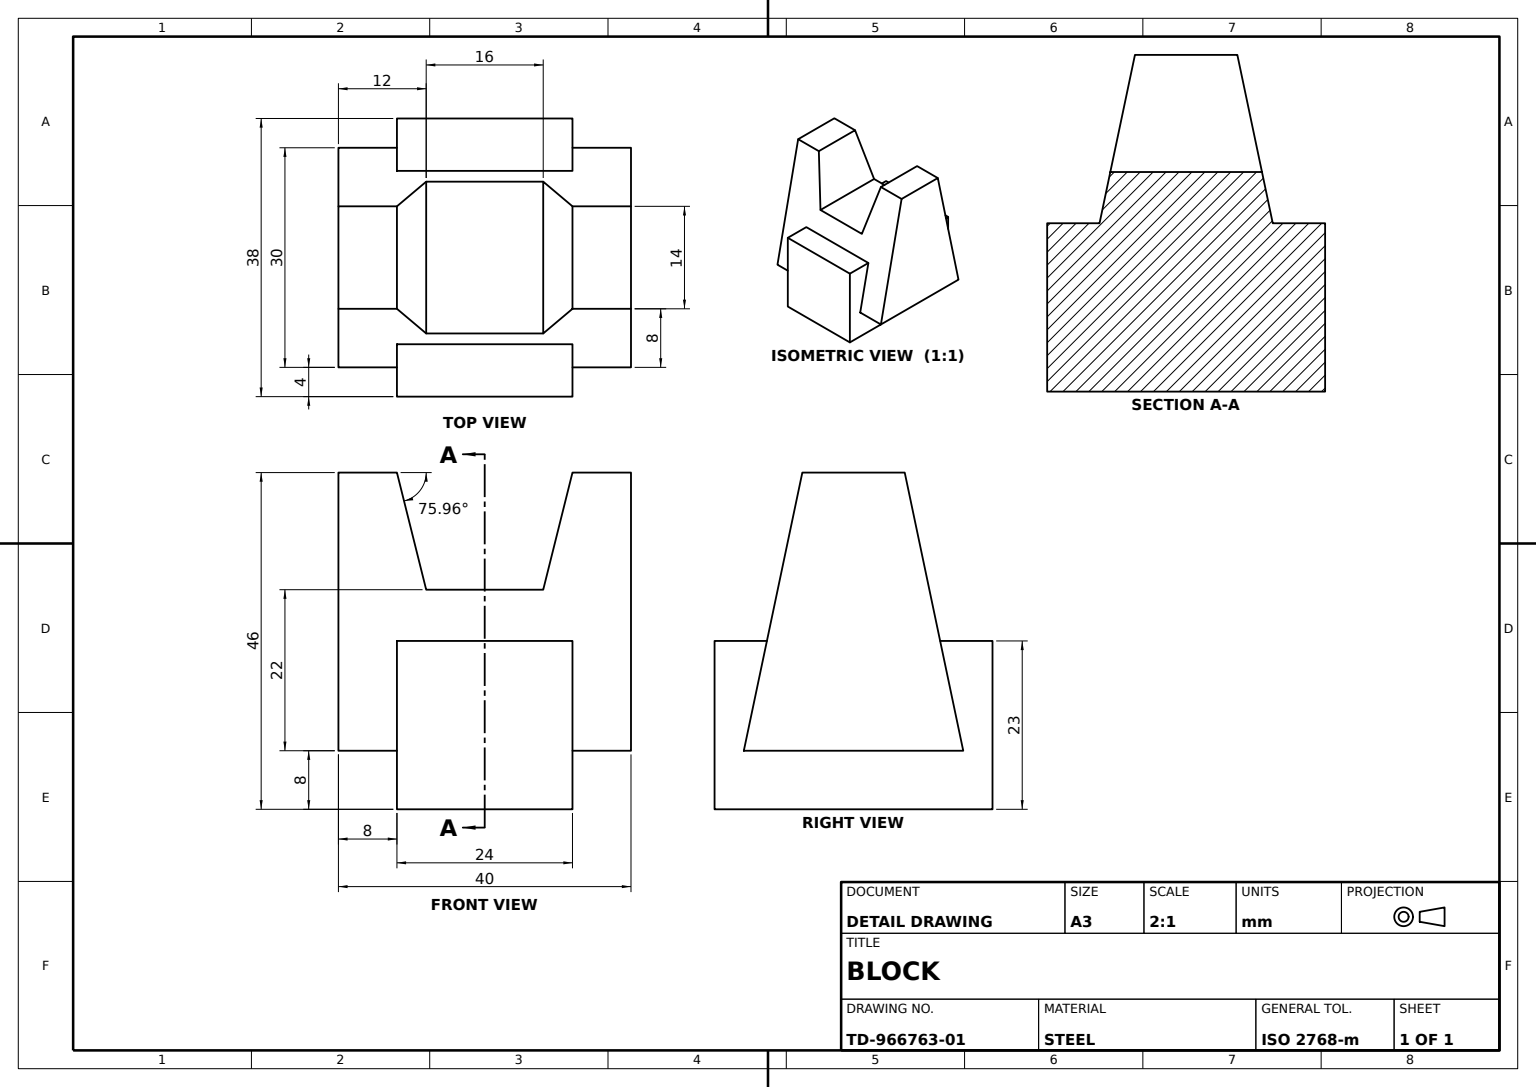
from build123d import *

# Parameters (mm, degrees)
BASE_BLOCK_30MM_DEPTH  = 15
GROOVE_CUT_40MM_DEPTH  = 20
FRONT_BLOCK_SKETCH_W   = 24
FRONT_BLOCK_SKETCH_H   = 23
FRONT_BLOCK_38MM_DEPTH = 19


with BuildPart() as part:
    # Base Profile Sketch → Base Block 30mm (new, symmetric)
    with BuildSketch(Plane.XY):
        Polygon((8, 22), (12, 38), (20, 38), (20, 0), (0, 0), (-20, 0), (-20, 38), (-12, 38), (-8, 22), align=None)
    extrude(amount=BASE_BLOCK_30MM_DEPTH, both=True)

    # Groove Profile Sketch → Groove Cut 40mm (cut, symmetric)
    with BuildSketch(Plane(origin=(0, 0, 0), x_dir=(0, 0, -1), z_dir=(1, 0, 0))):
        Polygon((-15, 0), (-7, 38), (-15, 38), align=None)
        Polygon((15, 38), (15, 0), (7, 38), align=None)
    extrude(amount=GROOVE_CUT_40MM_DEPTH, both=True, mode=Mode.SUBTRACT)

    # Front Block Sketch → Front Block 38mm (add, symmetric)
    with BuildSketch(Plane.XY):
        with Locations((0, 3.5)):
            Rectangle(FRONT_BLOCK_SKETCH_W, FRONT_BLOCK_SKETCH_H)
    extrude(amount=FRONT_BLOCK_38MM_DEPTH, both=True)


solid = part.part
